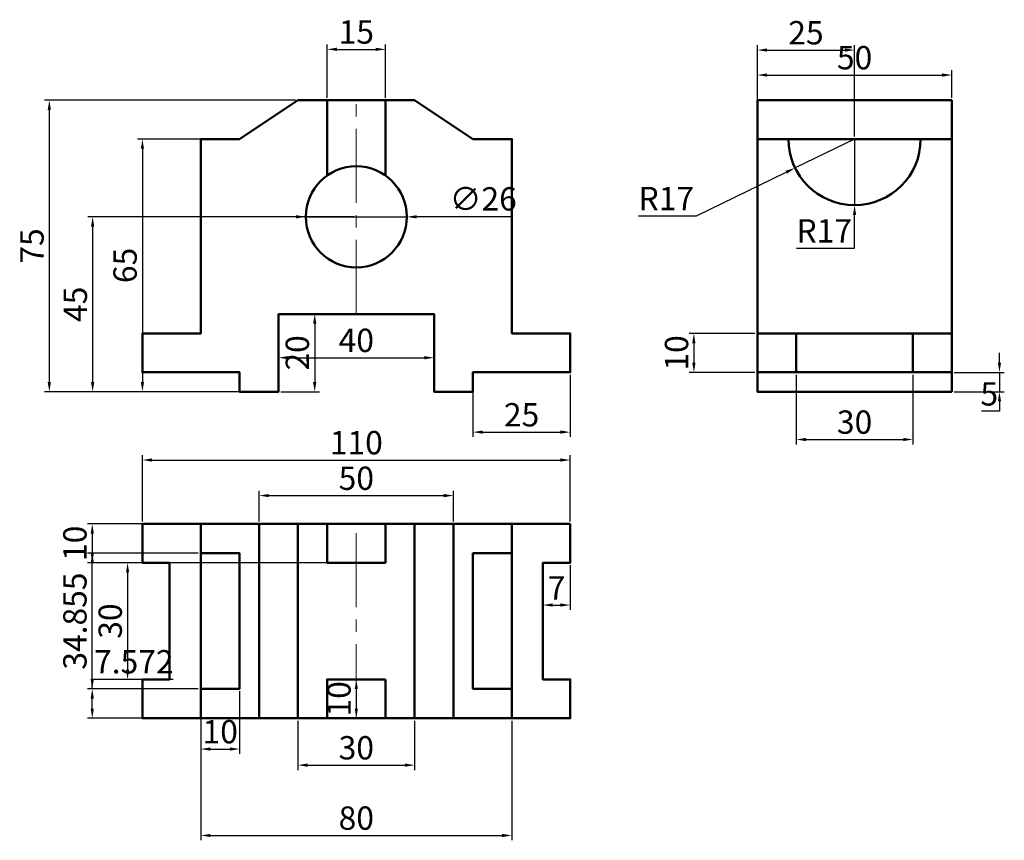
# Model space of a CAD drawing. Units: millimetres. Extents: x 97 to 350, y 23 to 234.
import ezdxf

# ---------------------------------------------------------------- set-up
doc = ezdxf.new("R2010")
doc.units = ezdxf.units.MM
doc.linetypes.add('CENTER2', pattern=[28.575, 19.05, -3.175, 3.175, -3.175])
for name, color, linetype, lineweight in [('M-CNTR', 1, 'CENTER2', 18), ('M-DIMS', 2, 'Continuous', 25), ('M-OUTL', 7, 'Continuous', 50)]:
    doc.layers.add(name, color=color, linetype=linetype, lineweight=lineweight)
doc.styles.get("Standard").update_dxf_attribs({"font": 'arial.ttf'})
doc.dimstyles.new('ISO-25', dxfattribs={"dimtxt": 6, "dimasz": 2.5, "dimexe": 1.25, "dimexo": 0.625, "dimtad": 1, "dimtoh": 1, "dimdec": 0, "dimtxsty": 'Standard', "dimcen": 2.5, "dimadec": 0, "dimazin": 0, "dimtfac": 1, "dimtdec": 0, "dimtmove": 0, "dimatfit": 3, "dimfxl": 1, "dimarcsym": 0})

# ---------------------------------------------------------------- blocks, each defined once
blk = doc.blocks.new('*D1')
at = {"layer": 'Defpoints', "color": 0, "transparency": 16777216}
for p in [(163.24, 157.92), (163.24, 137.92), (172.54, 137.92)]:
    blk.add_point(p, dxfattribs=at)
at = {"layer": 'M-DIMS', "color": 0, "lineweight": -2, "transparency": 16777216}
for p, q in [((163.86, 157.92), (173.79, 157.92)), ((172.54, 155.42), (172.54, 140.42)), ((163.86, 137.92), (173.79, 137.92))]:
    blk.add_line(p, q, dxfattribs=at)
at = {"layer": 'M-DIMS', "color": 0, "transparency": 16777216}
for points in [[(172.12, 155.42), (172.96, 155.42), (172.54, 157.92)], [(172.12, 140.42), (172.96, 140.42), (172.54, 137.92)]]:
    blk.add_solid(points, dxfattribs=at)
at = {"layer": 'M-DIMS', "color": 0, "transparency": 16777216, "insert": (168.85, 147.92), "char_height": 6, "attachment_point": 5, "rotation": 90}
blk.add_mtext('20', dxfattribs=at)
blk = doc.blocks.new('*D2')
at = {"layer": 'Defpoints', "color": 0, "transparency": 16777216}
for p in [(163.24, 157.92), (203.24, 157.92), (203.24, 146.68)]:
    blk.add_point(p, dxfattribs=at)
at = {"layer": 'M-DIMS', "color": 0, "lineweight": -2, "transparency": 16777216}
for p, q in [((163.24, 157.3), (163.24, 145.43)), ((203.24, 157.3), (203.24, 145.43)), ((165.74, 146.68), (200.74, 146.68))]:
    blk.add_line(p, q, dxfattribs=at)
at = {"layer": 'M-DIMS', "color": 0, "transparency": 16777216}
for points in [[(165.74, 147.1), (165.74, 146.26), (163.24, 146.68)], [(200.74, 147.1), (200.74, 146.26), (203.24, 146.68)]]:
    blk.add_solid(points, dxfattribs=at)
at = {"layer": 'M-DIMS', "color": 0, "transparency": 16777216, "insert": (183.24, 150.37), "char_height": 6, "attachment_point": 5}
blk.add_mtext('40', dxfattribs=at)
blk = doc.blocks.new('*D3')
at = {"layer": 'Defpoints', "color": 0, "transparency": 16777216}
for p in [(213.24, 142.92), (238.24, 142.92), (238.24, 127.54)]:
    blk.add_point(p, dxfattribs=at)
at = {"layer": 'M-DIMS', "color": 0, "lineweight": -2, "transparency": 16777216}
for p, q in [((213.24, 142.3), (213.24, 126.29)), ((238.24, 142.3), (238.24, 126.29)), ((215.74, 127.54), (235.74, 127.54))]:
    blk.add_line(p, q, dxfattribs=at)
at = {"layer": 'M-DIMS', "color": 0, "transparency": 16777216}
for points in [[(215.74, 127.96), (215.74, 127.13), (213.24, 127.54)], [(235.74, 127.96), (235.74, 127.13), (238.24, 127.54)]]:
    blk.add_solid(points, dxfattribs=at)
at = {"layer": 'M-DIMS', "color": 0, "transparency": 16777216, "insert": (225.74, 131.23), "char_height": 6, "attachment_point": 5}
blk.add_mtext('25', dxfattribs=at)
blk = doc.blocks.new('*D4')
at = {"layer": 'Defpoints', "color": 0, "transparency": 16777216}
for p in [(190.74, 226.01), (175.74, 212.92), (190.74, 212.92)]:
    blk.add_point(p, dxfattribs=at)
at = {"layer": 'M-DIMS', "color": 0, "lineweight": -2, "transparency": 16777216}
for p, q in [((175.74, 213.55), (175.74, 227.26)), ((178.24, 226.01), (188.24, 226.01)), ((190.74, 213.55), (190.74, 227.26))]:
    blk.add_line(p, q, dxfattribs=at)
at = {"layer": 'M-DIMS', "color": 0, "transparency": 16777216}
for points in [[(178.24, 226.43), (178.24, 225.6), (175.74, 226.01)], [(188.24, 226.43), (188.24, 225.6), (190.74, 226.01)]]:
    blk.add_solid(points, dxfattribs=at)
at = {"layer": 'M-DIMS', "color": 0, "transparency": 16777216, "insert": (183.24, 229.7), "char_height": 6, "attachment_point": 5}
blk.add_mtext('15', dxfattribs=at)
blk = doc.blocks.new('*D5')
at = {"layer": 'Defpoints', "color": 0, "transparency": 16777216}
for p in [(183.24, 182.92), (115.43, 137.92), (163.24, 137.92)]:
    blk.add_point(p, dxfattribs=at)
at = {"layer": 'M-DIMS', "color": 0, "lineweight": -2, "transparency": 16777216}
for p, q in [((182.61, 182.92), (114.18, 182.92)), ((115.43, 180.42), (115.43, 140.42)), ((162.61, 137.92), (114.18, 137.92))]:
    blk.add_line(p, q, dxfattribs=at)
at = {"layer": 'M-DIMS', "color": 0, "transparency": 16777216}
for points in [[(115.01, 180.42), (115.85, 180.42), (115.43, 182.92)], [(115.01, 140.42), (115.85, 140.42), (115.43, 137.92)]]:
    blk.add_solid(points, dxfattribs=at)
at = {"layer": 'M-DIMS', "color": 0, "transparency": 16777216, "insert": (111.75, 160.42), "char_height": 6, "attachment_point": 5, "rotation": 90}
blk.add_mtext('45', dxfattribs=at)
blk = doc.blocks.new('*D6')
at = {"layer": 'Defpoints', "color": 0, "transparency": 16777216}
for p in [(153.24, 202.92), (128.24, 137.92), (153.24, 137.92)]:
    blk.add_point(p, dxfattribs=at)
at = {"layer": 'M-DIMS', "color": 0, "lineweight": -2, "transparency": 16777216}
for p, q in [((152.61, 202.92), (126.99, 202.92)), ((128.24, 200.42), (128.24, 140.42)), ((152.61, 137.92), (126.99, 137.92))]:
    blk.add_line(p, q, dxfattribs=at)
at = {"layer": 'M-DIMS', "color": 0, "transparency": 16777216}
for points in [[(127.82, 200.42), (128.65, 200.42), (128.24, 202.92)], [(127.82, 140.42), (128.65, 140.42), (128.24, 137.92)]]:
    blk.add_solid(points, dxfattribs=at)
at = {"layer": 'M-DIMS', "color": 0, "transparency": 16777216, "insert": (124.55, 170.42), "char_height": 6, "attachment_point": 5, "rotation": 90}
blk.add_mtext('65', dxfattribs=at)
blk = doc.blocks.new('*D7')
at = {"layer": 'Defpoints', "color": 0, "transparency": 16777216}
for p in [(168.24, 212.92), (104.29, 137.92), (163.24, 137.92)]:
    blk.add_point(p, dxfattribs=at)
at = {"layer": 'M-DIMS', "color": 0, "lineweight": -2, "transparency": 16777216}
for p, q in [((167.61, 212.92), (103.04, 212.92)), ((104.29, 210.42), (104.29, 140.42)), ((162.61, 137.92), (103.04, 137.92))]:
    blk.add_line(p, q, dxfattribs=at)
at = {"layer": 'M-DIMS', "color": 0, "transparency": 16777216}
for points in [[(103.87, 210.42), (104.7, 210.42), (104.29, 212.92)], [(103.87, 140.42), (104.7, 140.42), (104.29, 137.92)]]:
    blk.add_solid(points, dxfattribs=at)
at = {"layer": 'M-DIMS', "color": 0, "transparency": 16777216, "insert": (100.61, 175.42), "char_height": 6, "attachment_point": 5, "rotation": 90}
blk.add_mtext('75', dxfattribs=at)
blk = doc.blocks.new('*D8')
at = {"layer": 'Defpoints', "color": 0, "transparency": 16777216}
for p in [(336.37, 219.4), (286.37, 212.92), (336.37, 212.92)]:
    blk.add_point(p, dxfattribs=at)
at = {"layer": 'M-DIMS', "color": 0, "lineweight": -2, "transparency": 16777216}
for p, q in [((286.37, 213.55), (286.37, 220.65)), ((336.37, 213.55), (336.37, 220.65)), ((288.87, 219.4), (333.87, 219.4))]:
    blk.add_line(p, q, dxfattribs=at)
at = {"layer": 'M-DIMS', "color": 0, "transparency": 16777216}
for points in [[(288.87, 219.82), (288.87, 218.99), (286.37, 219.4)], [(333.87, 219.82), (333.87, 218.99), (336.37, 219.4)]]:
    blk.add_solid(points, dxfattribs=at)
at = {"layer": 'M-DIMS', "color": 0, "transparency": 16777216, "insert": (311.37, 223.09), "char_height": 6, "attachment_point": 5}
blk.add_mtext('50', dxfattribs=at)
blk = doc.blocks.new('*D9')
at = {"layer": 'Defpoints', "color": 0, "transparency": 16777216}
for p in [(311.37, 202.92), (296.07, 195.5)]:
    blk.add_point(p, dxfattribs=at)
at = {"layer": 'M-DIMS', "color": 0, "lineweight": -2, "transparency": 16777216}
for p, q in [((311.37, 202.92), (296.07, 195.5)), ((270.74, 183.22), (293.82, 194.41)), ((255.78, 183.22), (270.74, 183.22))]:
    blk.add_line(p, q, dxfattribs=at)
at = {"layer": 'M-DIMS', "color": 0, "transparency": 16777216}
blk.add_solid([(293.64, 194.79), (294, 194.04), (296.07, 195.5)], dxfattribs=at)
at = {"layer": 'M-DIMS', "color": 0, "transparency": 16777216, "insert": (262.95, 186.85), "char_height": 6, "attachment_point": 5}
blk.add_mtext('R17', dxfattribs=at)
blk = doc.blocks.new('*D10')
at = {"layer": 'Defpoints', "color": 0, "transparency": 16777216}
for p in [(286.37, 152.92), (270.05, 142.92), (286.37, 142.92)]:
    blk.add_point(p, dxfattribs=at)
at = {"layer": 'M-DIMS', "color": 0, "lineweight": -2, "transparency": 16777216}
for p, q in [((285.74, 152.92), (268.8, 152.92)), ((270.05, 150.42), (270.05, 145.42)), ((285.74, 142.92), (268.8, 142.92))]:
    blk.add_line(p, q, dxfattribs=at)
at = {"layer": 'M-DIMS', "color": 0, "transparency": 16777216}
for points in [[(269.63, 150.42), (270.46, 150.42), (270.05, 152.92)], [(269.63, 145.42), (270.46, 145.42), (270.05, 142.92)]]:
    blk.add_solid(points, dxfattribs=at)
at = {"layer": 'M-DIMS', "color": 0, "transparency": 16777216, "insert": (266.36, 147.92), "char_height": 6, "attachment_point": 5, "rotation": 90}
blk.add_mtext('10', dxfattribs=at)
blk = doc.blocks.new('*D11')
at = {"layer": 'Defpoints', "color": 0, "transparency": 16777216}
for p in [(296.37, 142.92), (326.37, 142.92), (326.37, 125.64)]:
    blk.add_point(p, dxfattribs=at)
at = {"layer": 'M-DIMS', "color": 0, "lineweight": -2, "transparency": 16777216}
for p, q in [((296.37, 142.3), (296.37, 124.39)), ((326.37, 142.3), (326.37, 124.39)), ((298.87, 125.64), (323.87, 125.64))]:
    blk.add_line(p, q, dxfattribs=at)
at = {"layer": 'M-DIMS', "color": 0, "transparency": 16777216}
for points in [[(298.87, 126.06), (298.87, 125.23), (296.37, 125.64)], [(323.87, 126.06), (323.87, 125.23), (326.37, 125.64)]]:
    blk.add_solid(points, dxfattribs=at)
at = {"layer": 'M-DIMS', "color": 0, "transparency": 16777216, "insert": (311.37, 129.34), "char_height": 6, "attachment_point": 5}
blk.add_mtext('30', dxfattribs=at)
blk = doc.blocks.new('*D12')
at = {"layer": 'Defpoints', "color": 0, "transparency": 16777216}
for p in [(336.37, 142.92), (336.37, 137.92), (348.63, 137.92)]:
    blk.add_point(p, dxfattribs=at)
at = {"layer": 'M-DIMS', "color": 0, "lineweight": -2, "transparency": 16777216}
for p, q in [((348.63, 145.42), (348.63, 147.92)), ((336.99, 142.92), (349.88, 142.92)), ((348.63, 142.92), (348.63, 137.92)), ((336.99, 137.92), (349.88, 137.92)), ((348.63, 135.42), (348.63, 132.92)), ((348.63, 132.92), (344.02, 132.92))]:
    blk.add_line(p, q, dxfattribs=at)
at = {"layer": 'M-DIMS', "color": 0, "transparency": 16777216}
for points in [[(348.21, 145.42), (349.04, 145.42), (348.63, 142.92)], [(348.21, 135.42), (349.04, 135.42), (348.63, 137.92)]]:
    blk.add_solid(points, dxfattribs=at)
at = {"layer": 'M-DIMS', "color": 0, "transparency": 16777216, "insert": (346.01, 136.6), "char_height": 6, "attachment_point": 5}
blk.add_mtext('5', dxfattribs=at)
blk = doc.blocks.new('*D13')
at = {"layer": 'Defpoints', "color": 0, "transparency": 16777216}
for p in [(238.24, 120.36), (128.24, 103.93), (238.24, 103.93)]:
    blk.add_point(p, dxfattribs=at)
at = {"layer": 'M-DIMS', "color": 0, "lineweight": -2, "transparency": 16777216}
for p, q in [((128.24, 104.56), (128.24, 121.61)), ((238.24, 104.56), (238.24, 121.61)), ((130.74, 120.36), (235.74, 120.36))]:
    blk.add_line(p, q, dxfattribs=at)
at = {"layer": 'M-DIMS', "color": 0, "transparency": 16777216}
for points in [[(130.74, 120.78), (130.74, 119.95), (128.24, 120.36)], [(235.74, 120.78), (235.74, 119.95), (238.24, 120.36)]]:
    blk.add_solid(points, dxfattribs=at)
at = {"layer": 'M-DIMS', "color": 0, "transparency": 16777216, "insert": (183.24, 124.05), "char_height": 6, "attachment_point": 5}
blk.add_mtext('110', dxfattribs=at)
blk = doc.blocks.new('*D14')
at = {"layer": 'Defpoints', "color": 0, "transparency": 16777216}
for p in [(208.24, 111.21), (158.24, 103.93), (208.24, 103.93)]:
    blk.add_point(p, dxfattribs=at)
at = {"layer": 'M-DIMS', "color": 0, "lineweight": -2, "transparency": 16777216}
for p, q in [((158.24, 104.56), (158.24, 112.46)), ((208.24, 104.56), (208.24, 112.46)), ((160.74, 111.21), (205.74, 111.21))]:
    blk.add_line(p, q, dxfattribs=at)
at = {"layer": 'M-DIMS', "color": 0, "transparency": 16777216}
for points in [[(160.74, 111.63), (160.74, 110.8), (158.24, 111.21)], [(205.74, 111.63), (205.74, 110.8), (208.24, 111.21)]]:
    blk.add_solid(points, dxfattribs=at)
at = {"layer": 'M-DIMS', "color": 0, "transparency": 16777216, "insert": (183.24, 114.9), "char_height": 6, "attachment_point": 5}
blk.add_mtext('50', dxfattribs=at)
blk = doc.blocks.new('*D15')
at = {"layer": 'Defpoints', "color": 0, "transparency": 16777216}
for p in [(175.74, 63.93), (175.74, 53.93), (183.24, 53.93)]:
    blk.add_point(p, dxfattribs=at)
at = {"layer": 'M-DIMS', "color": 0, "lineweight": -2, "transparency": 16777216}
for p, q in [((176.36, 63.93), (184.49, 63.93)), ((183.24, 61.43), (183.24, 56.43)), ((176.36, 53.93), (184.49, 53.93))]:
    blk.add_line(p, q, dxfattribs=at)
at = {"layer": 'M-DIMS', "color": 0, "transparency": 16777216}
for points in [[(182.82, 61.43), (183.65, 61.43), (183.24, 63.93)], [(182.82, 56.43), (183.65, 56.43), (183.24, 53.93)]]:
    blk.add_solid(points, dxfattribs=at)
at = {"layer": 'M-DIMS', "color": 0, "transparency": 16777216, "insert": (179.55, 58.93), "char_height": 6, "attachment_point": 5, "rotation": 90}
blk.add_mtext('10', dxfattribs=at)
blk = doc.blocks.new('*D16')
at = {"layer": 'Defpoints', "color": 0, "transparency": 16777216}
for p in [(143.24, 61.5), (153.24, 61.5), (153.24, 46.01)]:
    blk.add_point(p, dxfattribs=at)
at = {"layer": 'M-DIMS', "color": 0, "lineweight": -2, "transparency": 16777216}
for p, q in [((143.24, 60.88), (143.24, 44.76)), ((153.24, 60.88), (153.24, 44.76)), ((145.74, 46.01), (150.74, 46.01))]:
    blk.add_line(p, q, dxfattribs=at)
at = {"layer": 'M-DIMS', "color": 0, "transparency": 16777216}
for points in [[(145.74, 46.43), (145.74, 45.59), (143.24, 46.01)], [(150.74, 46.43), (150.74, 45.59), (153.24, 46.01)]]:
    blk.add_solid(points, dxfattribs=at)
at = {"layer": 'M-DIMS', "color": 0, "transparency": 16777216, "insert": (148.24, 49.7), "char_height": 6, "attachment_point": 5}
blk.add_mtext('10', dxfattribs=at)
blk = doc.blocks.new('*D17')
at = {"layer": 'Defpoints', "color": 0, "transparency": 16777216}
for p in [(168.24, 53.93), (198.24, 53.93), (198.24, 41.87)]:
    blk.add_point(p, dxfattribs=at)
at = {"layer": 'M-DIMS', "color": 0, "lineweight": -2, "transparency": 16777216}
for p, q in [((168.24, 53.31), (168.24, 40.62)), ((198.24, 53.31), (198.24, 40.62)), ((170.74, 41.87), (195.74, 41.87))]:
    blk.add_line(p, q, dxfattribs=at)
at = {"layer": 'M-DIMS', "color": 0, "transparency": 16777216}
for points in [[(170.74, 42.29), (170.74, 41.45), (168.24, 41.87)], [(195.74, 42.29), (195.74, 41.45), (198.24, 41.87)]]:
    blk.add_solid(points, dxfattribs=at)
at = {"layer": 'M-DIMS', "color": 0, "transparency": 16777216, "insert": (183.24, 45.56), "char_height": 6, "attachment_point": 5}
blk.add_mtext('30', dxfattribs=at)
blk = doc.blocks.new('*D18')
at = {"layer": 'Defpoints', "color": 0, "transparency": 16777216}
for p in [(143.24, 53.93), (223.24, 53.93), (223.24, 23.78)]:
    blk.add_point(p, dxfattribs=at)
at = {"layer": 'M-DIMS', "color": 0, "lineweight": -2, "transparency": 16777216}
for p, q in [((143.24, 53.31), (143.24, 22.53)), ((223.24, 53.31), (223.24, 22.53)), ((145.74, 23.78), (220.74, 23.78))]:
    blk.add_line(p, q, dxfattribs=at)
at = {"layer": 'M-DIMS', "color": 0, "transparency": 16777216}
for points in [[(145.74, 24.2), (145.74, 23.37), (143.24, 23.78)], [(220.74, 24.2), (220.74, 23.37), (223.24, 23.78)]]:
    blk.add_solid(points, dxfattribs=at)
at = {"layer": 'M-DIMS', "color": 0, "transparency": 16777216, "insert": (183.24, 27.47), "char_height": 6, "attachment_point": 5}
blk.add_mtext('80', dxfattribs=at)
blk = doc.blocks.new('*D19')
at = {"layer": 'Defpoints', "color": 0, "transparency": 16777216}
for p in [(231.24, 93.93), (238.24, 93.93), (238.24, 83.06)]:
    blk.add_point(p, dxfattribs=at)
at = {"layer": 'M-DIMS', "color": 0, "lineweight": -2, "transparency": 16777216}
for p, q in [((231.24, 93.31), (231.24, 81.81)), ((238.24, 93.31), (238.24, 81.81)), ((233.74, 83.06), (235.74, 83.06))]:
    blk.add_line(p, q, dxfattribs=at)
at = {"layer": 'M-DIMS', "color": 0, "transparency": 16777216}
for points in [[(233.74, 83.47), (233.74, 82.64), (231.24, 83.06)], [(235.74, 83.47), (235.74, 82.64), (238.24, 83.06)]]:
    blk.add_solid(points, dxfattribs=at)
at = {"layer": 'M-DIMS', "color": 0, "transparency": 16777216, "insert": (234.74, 86.68), "char_height": 6, "attachment_point": 5}
blk.add_mtext('7', dxfattribs=at)
blk = doc.blocks.new('*D20')
at = {"layer": 'Defpoints', "color": 0, "transparency": 16777216}
for p in [(128.24, 93.93), (124.42, 63.93), (128.24, 63.93)]:
    blk.add_point(p, dxfattribs=at)
at = {"layer": 'M-DIMS', "color": 0, "lineweight": -2, "transparency": 16777216}
for p, q in [((127.61, 93.93), (123.17, 93.93)), ((124.42, 91.43), (124.42, 66.43)), ((127.61, 63.93), (123.17, 63.93))]:
    blk.add_line(p, q, dxfattribs=at)
at = {"layer": 'M-DIMS', "color": 0, "transparency": 16777216}
for points in [[(124, 91.43), (124.83, 91.43), (124.42, 93.93)], [(124, 66.43), (124.83, 66.43), (124.42, 63.93)]]:
    blk.add_solid(points, dxfattribs=at)
at = {"layer": 'M-DIMS', "color": 0, "transparency": 16777216, "insert": (120.73, 78.93), "char_height": 6, "attachment_point": 5, "rotation": 90}
blk.add_mtext('30', dxfattribs=at)
blk = doc.blocks.new('*D21')
at = {"layer": 'Defpoints', "color": 0, "transparency": 16777216}
for p in [(115.34, 96.36), (143.24, 96.36), (143.24, 61.5)]:
    blk.add_point(p, dxfattribs=at)
at = {"layer": 'M-DIMS', "color": 0, "lineweight": -2, "transparency": 16777216}
for p, q in [((142.61, 96.36), (114.09, 96.36)), ((115.34, 64), (115.34, 93.86)), ((142.61, 61.5), (114.09, 61.5))]:
    blk.add_line(p, q, dxfattribs=at)
at = {"layer": 'M-DIMS', "color": 0, "transparency": 16777216}
for points in [[(114.92, 93.86), (115.75, 93.86), (115.34, 96.36)], [(114.92, 64), (115.75, 64), (115.34, 61.5)]]:
    blk.add_solid(points, dxfattribs=at)
at = {"layer": 'M-DIMS', "color": 0, "transparency": 16777216, "insert": (111.65, 78.93), "char_height": 6, "attachment_point": 5, "rotation": 90}
blk.add_mtext('34.855', dxfattribs=at)
blk = doc.blocks.new('*D22')
at = {"layer": 'Defpoints', "color": 0, "transparency": 16777216}
for p in [(115.34, 61.5), (143.24, 61.5), (143.24, 53.93)]:
    blk.add_point(p, dxfattribs=at)
at = {"layer": 'M-DIMS', "color": 0, "lineweight": -2, "transparency": 16777216}
for p, q in [((115.34, 61.5), (115.34, 64)), ((115.34, 64), (136.1, 64)), ((142.61, 61.5), (114.09, 61.5)), ((115.34, 56.43), (115.34, 59)), ((142.61, 53.93), (114.09, 53.93))]:
    blk.add_line(p, q, dxfattribs=at)
at = {"layer": 'M-DIMS', "color": 0, "transparency": 16777216}
for points in [[(114.92, 59), (115.75, 59), (115.34, 61.5)], [(114.92, 56.43), (115.75, 56.43), (115.34, 53.93)]]:
    blk.add_solid(points, dxfattribs=at)
at = {"layer": 'M-DIMS', "color": 0, "transparency": 16777216, "insert": (126.03, 67.69), "char_height": 6, "attachment_point": 5}
blk.add_mtext('7.572', dxfattribs=at)
blk = doc.blocks.new('*D23')
at = {"layer": 'Defpoints', "color": 0, "transparency": 16777216}
for p in [(190.74, 103.93), (115.34, 93.93), (190.74, 93.93)]:
    blk.add_point(p, dxfattribs=at)
at = {"layer": 'M-DIMS', "color": 0, "lineweight": -2, "transparency": 16777216}
for p, q in [((190.11, 103.93), (114.09, 103.93)), ((115.34, 101.43), (115.34, 96.43)), ((190.11, 93.93), (114.09, 93.93))]:
    blk.add_line(p, q, dxfattribs=at)
at = {"layer": 'M-DIMS', "color": 0, "transparency": 16777216}
for points in [[(114.92, 101.43), (115.75, 101.43), (115.34, 103.93)], [(114.92, 96.43), (115.75, 96.43), (115.34, 93.93)]]:
    blk.add_solid(points, dxfattribs=at)
at = {"layer": 'M-DIMS', "color": 0, "transparency": 16777216, "insert": (111.65, 98.93), "char_height": 6, "attachment_point": 5, "rotation": 90}
blk.add_mtext('10', dxfattribs=at)
blk = doc.blocks.new('*D24')
at = {"layer": 'Defpoints', "color": 0, "transparency": 16777216}
for p in [(311.37, 225.82), (286.37, 202.92), (311.37, 202.92)]:
    blk.add_point(p, dxfattribs=at)
at = {"layer": 'M-DIMS', "color": 0, "lineweight": -2, "transparency": 16777216}
for p, q in [((286.37, 203.55), (286.37, 227.07)), ((288.87, 225.82), (308.87, 225.82)), ((311.37, 203.55), (311.37, 227.07))]:
    blk.add_line(p, q, dxfattribs=at)
at = {"layer": 'M-DIMS', "color": 0, "transparency": 16777216}
for points in [[(288.87, 226.24), (288.87, 225.41), (286.37, 225.82)], [(308.87, 226.24), (308.87, 225.41), (311.37, 225.82)]]:
    blk.add_solid(points, dxfattribs=at)
at = {"layer": 'M-DIMS', "color": 0, "transparency": 16777216, "insert": (298.87, 229.51), "char_height": 6, "attachment_point": 5}
blk.add_mtext('25', dxfattribs=at)
blk = doc.blocks.new('*D25')
at = {"layer": 'Defpoints', "color": 0, "transparency": 16777216}
for p in [(170.24, 182.93), (196.24, 182.92)]:
    blk.add_point(p, dxfattribs=at)
at = {"layer": 'M-DIMS', "color": 0, "lineweight": -2, "transparency": 16777216}
for p, q in [((167.74, 182.93), (165.24, 182.93)), ((170.24, 182.93), (196.24, 182.92)), ((207.7, 182.92), (198.74, 182.92)), ((223.44, 182.92), (207.7, 182.92))]:
    blk.add_line(p, q, dxfattribs=at)
at = {"layer": 'M-DIMS', "color": 0, "transparency": 16777216}
for points in [[(167.74, 183.35), (167.74, 182.51), (170.24, 182.93)], [(198.74, 183.34), (198.74, 182.5), (196.24, 182.92)]]:
    blk.add_solid(points, dxfattribs=at)
at = {"layer": 'M-DIMS', "color": 0, "transparency": 16777216, "insert": (215.88, 186.77), "char_height": 6, "attachment_point": 5}
blk.add_mtext('∅26', dxfattribs=at)
blk = doc.blocks.new('*D26')
at = {"layer": 'Defpoints', "color": 0, "transparency": 16777216}
for p in [(311.37, 202.92), (311.37, 185.92)]:
    blk.add_point(p, dxfattribs=at)
at = {"layer": 'M-DIMS', "color": 0, "lineweight": -2, "transparency": 16777216}
for p, q in [((311.37, 202.92), (311.37, 185.92)), ((311.37, 174.9), (311.37, 183.42)), ((296.4, 174.9), (311.37, 174.9))]:
    blk.add_line(p, q, dxfattribs=at)
at = {"layer": 'M-DIMS', "color": 0, "transparency": 16777216}
blk.add_solid([(310.95, 183.42), (311.78, 183.42), (311.37, 185.92)], dxfattribs=at)
at = {"layer": 'M-DIMS', "color": 0, "transparency": 16777216, "insert": (303.57, 178.54), "char_height": 6, "attachment_point": 5}
blk.add_mtext('R17', dxfattribs=at)

msp = doc.modelspace()

# ---------------------------------------------------------------- linework, layer by layer
at = {"layer": 'M-CNTR'}
for p, q in [((183.2372, 157.9248), (183.2372, 212.9248)), ((175.7372, 93.9316), (175.7372, 103.9316)), ((183.2372, 53.9316), (183.2372, 103.9316)), ((175.7372, 53.9316), (175.7372, 63.9316))]:
    msp.add_line(p, q, dxfattribs=at)
at = {"layer": 'M-OUTL'}
for p, q in [((336.3662, 202.9248), (286.3662, 202.9248)), ((326.3662, 202.9248), (296.3662, 202.9248)), ((286.3662, 152.9248), (336.3662, 152.9248)), ((296.3662, 152.9248), (296.3662, 142.9248)), ((326.3662, 142.9248), (326.3662, 152.9248)), ((286.3662, 142.9248), (336.3662, 142.9248)), ((143.2372, 53.9316), (143.2372, 103.9316)), ((158.2372, 53.9316), (158.2372, 103.9316)), ((168.2372, 53.9316), (168.2372, 103.9316)), ((190.7372, 93.9316), (190.7372, 103.9316)), ((198.2372, 53.9316), (198.2372, 103.9316)), ((208.2372, 53.9316), (208.2372, 103.9316)), ((223.2372, 53.9316), (223.2372, 103.9316)), ((135.2372, 93.9316), (128.2372, 93.9316)), ((175.7372, 93.9316), (190.7372, 93.9316)), ((231.2372, 93.9316), (238.2372, 93.9316)), ((128.2372, 63.9316), (135.2372, 63.9316)), ((175.7372, 63.9316), (190.7372, 63.9316)), ((190.7372, 53.9316), (190.7372, 63.9316)), ((231.2372, 63.9316), (238.2372, 63.9316))]:
    msp.add_line(p, q, dxfattribs=at)
for points in [[(175.7372, 193.5432), (175.7372, 212.9248), (168.2372, 212.9248), (153.2372, 202.9248), (143.2372, 202.9248), (143.2372, 152.9248), (128.2372, 152.9248), (128.2372, 142.9248), (153.2372, 142.9248), (153.2372, 137.9248), (163.2372, 137.9248), (163.2372, 157.9248), (203.2372, 157.9248), (203.2372, 137.9248), (213.2372, 137.9248), (213.2372, 142.9248), (238.2372, 142.9248), (238.2372, 152.9248), (223.2372, 152.9248), (223.2372, 202.9248), (213.2372, 202.9248), (198.2372, 212.9248), (190.7372, 212.9248), (190.7372, 193.5432)], [(175.7372, 212.9248), (183.2372, 212.9248), (190.7372, 212.9248)], [(143.2372, 61.5039), (153.2372, 61.5039), (153.2372, 96.3593), (143.2372, 96.3593)], [(223.2372, 61.5039), (213.2372, 61.5039), (213.2372, 96.3593), (223.2372, 96.3593)]]:
    msp.add_lwpolyline(points, dxfattribs=at)
for points in [[(336.3662, 137.9248), (336.3662, 212.9248), (286.3662, 212.9248), (286.3662, 137.9248)], [(238.2372, 103.9316), (238.2372, 93.9316), (231.2372, 93.9316), (231.2372, 63.9316), (238.2372, 63.9316), (238.2372, 53.9316), (128.2372, 53.9316), (128.2372, 63.9316), (135.2372, 63.9316), (135.2372, 93.9316), (128.2372, 93.9316), (128.2372, 103.9316)], [(175.7372, 93.9316), (175.7372, 103.9316)], [(175.7372, 53.9316), (175.7372, 63.9316)]]:
    msp.add_lwpolyline(points, close=True, dxfattribs=at)
msp.add_circle((183.2372, 182.9248), 13, dxfattribs=at)
msp.add_arc((311.3662, 202.9248), 17, 180, 0, dxfattribs=at)

# ---------------------------------------------------------------- dimensions: what is measured, and where the dimension line sits
at = {"layer": 'M-DIMS'}
for base, p1, p2, override, picture, middle in [((190.7372, 226.0141), (175.7372, 212.9248), (190.7372, 212.9248), {"dimclrd": 0, "dimclre": 0, "dimclrt": 0}, '*D4', (183.2372, 229.7025)), ((311.3662, 225.8248), (286.3662, 202.9248), (311.3662, 202.9248), {"dimdec": 0, "dimlfac": 1, "dimrnd": 0, "dimzin": 0, "dimdsep": 46, "dimlunit": 2}, '*D24', (298.8662, 229.5133)), ((336.3662, 219.4029), (286.3662, 212.9248), (336.3662, 212.9248), {"dimclrd": 0, "dimclre": 0, "dimclrt": 0}, '*D8', (311.3662, 223.0914)), ((203.2372, 146.6802), (163.2372, 157.9248), (203.2372, 157.9248), {"dimclrd": 0, "dimclre": 0, "dimclrt": 0}, '*D2', (183.2372, 150.3686)), ((238.2372, 127.5426), (213.2372, 142.9248), (238.2372, 142.9248), {"dimclrd": 0, "dimclre": 0, "dimclrt": 0}, '*D3', (225.7372, 131.231)), ((326.3662, 125.6448), (296.3662, 142.9248), (326.3662, 142.9248), {"dimclrd": 0, "dimclre": 0, "dimclrt": 0}, '*D11', (311.3662, 129.3353)), ((238.2372, 120.3648), (128.2372, 103.9316), (238.2372, 103.9316), {"dimclrd": 0, "dimclre": 0, "dimclrt": 0}, '*D13', (183.2372, 124.0532)), ((208.2372, 111.212), (158.2372, 103.9316), (208.2372, 103.9316), {"dimclrd": 0, "dimclre": 0, "dimclrt": 0}, '*D14', (183.2372, 114.9005)), ((238.2372, 83.0576), (231.2372, 93.9316), (238.2372, 93.9316), {"dimclrd": 0, "dimclre": 0, "dimclrt": 0}, '*D19', (234.7372, 86.6826)), ((153.2372, 46.0107), (143.2372, 61.5039), (153.2372, 61.5039), {"dimclrd": 0, "dimclre": 0, "dimclrt": 0}, '*D16', (148.2372, 49.6991)), ((223.2372, 23.7825), (143.2372, 53.9316), (223.2372, 53.9316), {"dimclrd": 0, "dimclre": 0, "dimclrt": 0}, '*D18', (183.2372, 27.4709)), ((198.2372, 41.8701), (168.2372, 53.9316), (198.2372, 53.9316), {"dimclrd": 0, "dimclre": 0, "dimclrt": 0}, '*D17', (183.2372, 45.5606))]:
    dim = msp.add_linear_dim(base=base, p1=p1, p2=p2, dimstyle='ISO-25', override=override, dxfattribs=at)
    dim.commit()
    dim.dimension.update_dxf_attribs({"geometry": picture, "text_midpoint": middle})
for base, p1, p2, override, picture, middle in [((104.2866, 137.9248), (168.2372, 212.9248), (163.2372, 137.9248), {"dimclrd": 0, "dimclre": 0, "dimclrt": 0}, '*D7', (100.6105, 175.4248)), ((128.2372, 137.9248), (153.2372, 202.9248), (153.2372, 137.9248), {"dimclrd": 0, "dimclre": 0, "dimclrt": 0}, '*D6', (124.5488, 170.4248)), ((115.4302, 137.9248), (183.2372, 182.9248), (163.2372, 137.9248), {"dimclrd": 0, "dimclre": 0, "dimclrt": 0}, '*D5', (111.7541, 160.4248)), ((172.5413, 137.9248), (163.2372, 157.9248), (163.2372, 137.9248), {"dimclrd": 0, "dimclre": 0, "dimclrt": 0}, '*D1', (168.8529, 147.9248)), ((270.0481, 142.9248), (286.3662, 152.9248), (286.3662, 142.9248), {"dimclrd": 0, "dimclre": 0, "dimclrt": 0}, '*D10', (266.3596, 147.9248)), ((348.6264, 137.9248), (336.3662, 142.9248), (336.3662, 137.9248), {"dimclrd": 0, "dimclre": 0, "dimclrt": 0}, '*D12', (346.0123, 136.601)), ((115.3372, 93.9316), (190.7372, 103.9316), (190.7372, 93.9316), {"dimdec": 0, "dimlfac": 1, "dimrnd": 0, "dimzin": 0, "dimdsep": 46, "dimlunit": 2}, '*D23', (111.6488, 98.9316)), ((115.3372, 96.3593), (143.2372, 61.5039), (143.2372, 96.3593), {"dimdec": 3, "dimlfac": 1, "dimrnd": 0, "dimzin": 0, "dimdsep": 46, "dimlunit": 2}, '*D21', (111.6467, 78.9316)), ((124.4162, 63.9316), (128.2372, 93.9316), (128.2372, 63.9316), {"dimclrd": 0, "dimclre": 0, "dimclrt": 0}, '*D20', (120.7257, 78.9316)), ((115.3372, 61.5039), (143.2372, 53.9316), (143.2372, 61.5039), {"dimdec": 3, "dimlfac": 1, "dimrnd": 0, "dimzin": 0, "dimdsep": 46, "dimlunit": 2}, '*D22', (126.0304, 67.6924)), ((183.2372, 53.9316), (175.7372, 63.9316), (175.7372, 53.9316), {"dimclrd": 0, "dimclre": 0, "dimclrt": 0}, '*D15', (179.5488, 58.9316))]:
    dim = msp.add_linear_dim(base=base, p1=p1, p2=p2, angle=90, dimstyle='ISO-25', override=override, dxfattribs=at)
    dim.commit()
    dim.dimension.update_dxf_attribs({"geometry": picture, "text_midpoint": middle})
dim = msp.add_radius_dim(center=(311.3662, 202.9248), mpoint=(296.0714, 195.5039), dimstyle='ISO-25', override={"dimclrd": 0, "dimclre": 0, "dimclrt": 0}, dxfattribs=at)
dim.commit()
dim.dimension.update_dxf_attribs({"geometry": '*D9', "text_midpoint": (262.9511, 183.2155), "dimtype": 164})
dim = msp.add_radius_dim(center=(311.3662, 202.9248), mpoint=(311.366, 185.9248), dimstyle='ISO-25', override={"dimdec": 0, "dimlfac": 1, "dimrnd": 0, "dimzin": 0, "dimdsep": 46, "dimlunit": 2}, dxfattribs=at)
dim.commit()
dim.dimension.update_dxf_attribs({"geometry": '*D26', "text_midpoint": (303.5724, 178.5375)})
dim = msp.add_diameter_dim_2p(p1=(170.2372, 182.9296), p2=(196.2372, 182.92), dimstyle='ISO-25', override={"dimdec": 0, "dimlfac": 1, "dimrnd": 0, "dimzin": 0, "dimdsep": 46, "dimlunit": 2}, dxfattribs=at)
dim.commit()
dim.dimension.update_dxf_attribs({"geometry": '*D25', "text_midpoint": (207.6997, 182.9158)})

doc.saveas('drawing.dxf')
